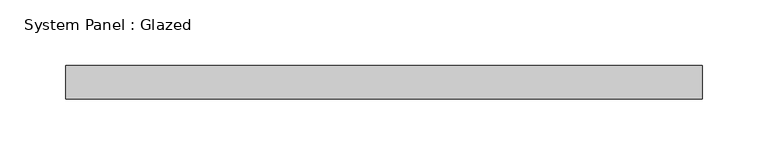
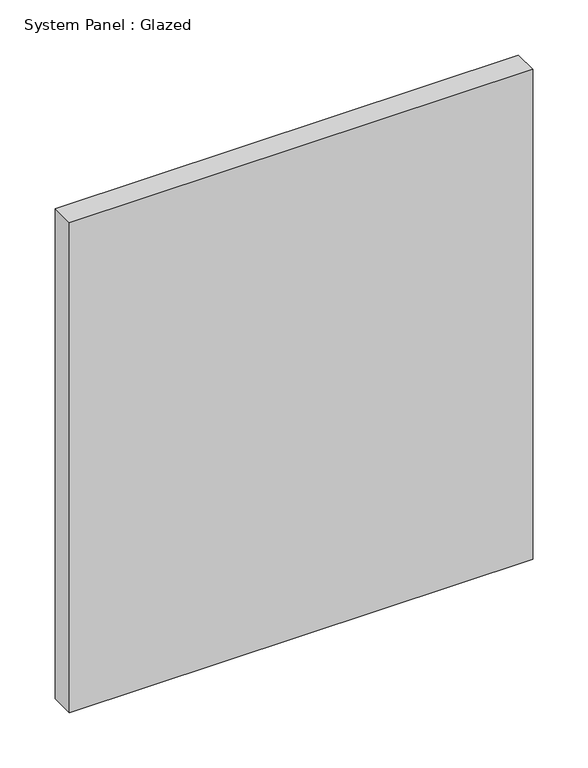
"""IFC4 building model written with IfcOpenShell, lengths in millimetres: plate geometry, System Panel : Glazed."""

from ifc_helpers import new_model, si_unit, origin, origin_with_axes, place, context, project, spatial, polyline, outline, extrude, source, transform, mapped, element, save


def system_panel_glazed_2a04ea5f(model_context):
    return source(origin(), model_context, "Body", "SweptSolid", [
        extrude(outline(polyline([(241.3, 19.05), (-241.3, 19.05), (-241.3, 44.45), (241.3, 44.45), (241.3, 19.05)])), origin_with_axes(), (0.0, 0.0, 1.0), 539.75),
    ])


if __name__ == "__main__":
    model = new_model("IFC4")
    model_context = context("Model", 3, world=origin())
    ifc_project = project(units=[si_unit("LENGTHUNIT", "METRE", prefix="MILLI")], contexts=[model_context])
    site = spatial("IfcSite", under=ifc_project)
    building = spatial("IfcBuilding", under=site)
    placement = place(None, origin())
    system_panel_glazed_shape = system_panel_glazed_2a04ea5f(model_context)
    element("IfcPlate", 1, ObjectType="System Panel : Glazed", at=placement, inside=building, context=model_context, shape_type="MappedRepresentation", body=[
        mapped(system_panel_glazed_shape, transform((0.0, 0.0, 0.0), x_axis=(1.0, 0.0, 0.0), y_axis=(0.0, 1.0, 0.0), z_axis=(0.0, 0.0, 1.0))),
    ])
    save(model, "model.ifc")

# Revit data of these elements
# Type "System Panel : Glazed"
#   Construction Type Id = "GSP4R"
#   Analytic Construction = "1/8 in Pilkington single glazing"
#   Visual Light Transmittance = 0.9
#   Solar Heat Gain Coefficient = 0.86
#   Heat Transfer Coefficient (U) = 1.18115 BTU/(h·ft²·°F)
#   Define Thermal Properties by = 1
# Element 1 (IfcPlate, "System Panel : Glazed")
#   Materials on its faces: "Glass"
# Materials
#   "Glass": class "Glass", colour RGB 0 128 192, transparency 0.75, Description = "Soda Lime Glass", Cost = 0
